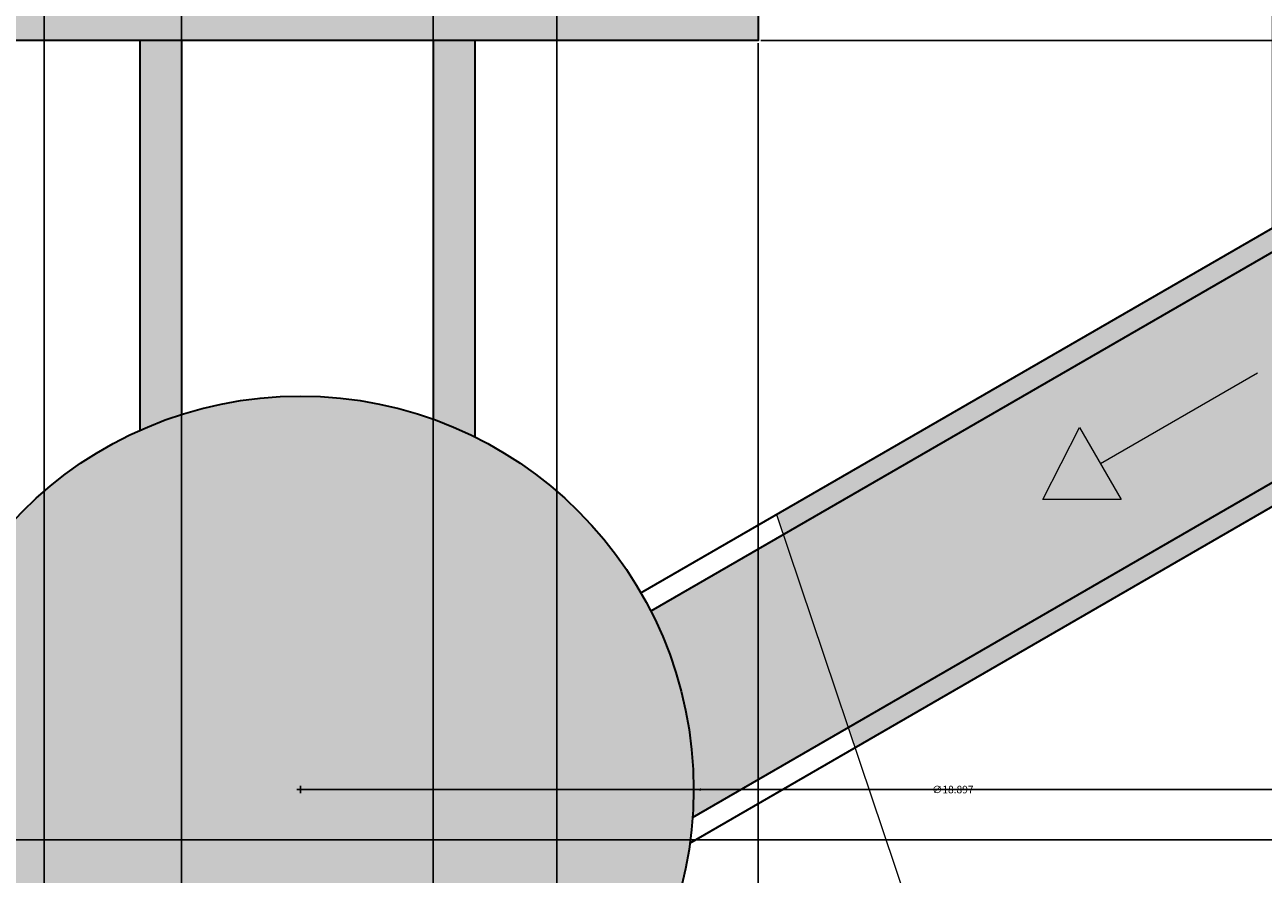
# Model space of a CAD drawing. Units: inches. Extents: x -1 to 292, y -3 to 199.
# Tile 44 of 52: x 237 to 267, y 43 to 63. Entities that reach past the tile are written whole.
import ezdxf

# ---------------------------------------------------------------- set-up
doc = ezdxf.new("R2010")
doc.units = ezdxf.units.IN
doc.header["$MEASUREMENT"] = 0
for name, color, linetype, lineweight in [('M-ANNO-LEAD', 2, 'Continuous', 18), ('M-ANNO-SYMB', 1, 'Continuous', 18), ('M-DIMS', 2, 'Continuous', 18), ('M-EQPM', 7, 'Continuous', 35), ('M-PATT', 8, 'Continuous', 13)]:
    doc.layers.add(name, color=color, linetype=linetype, lineweight=lineweight)
doc.styles.get("Standard").update_dxf_attribs({"font": 'arial.ttf'})
doc.dimstyles.get("Standard").update_dxf_attribs({"dimtxt": 0.18, "dimasz": 0.18, "dimexe": 0.18, "dimexo": 0.0625, "dimgap": 0.09, "dimtad": 0, "dimtih": 1, "dimtoh": 1, "dimdec": 4, "dimzin": 0, "dimdsep": 46, "dimtxsty": 'Standard', "dimcen": 0.09, "dimadec": 0, "dimazin": 0, "dimtfac": 1, "dimtdec": 4, "dimtofl": 0, "dimtmove": 0, "dimatfit": 3, "dimfxl": 1, "dimtolj": 1, "dimtzin": 0, "dimarcsym": 0})

# ---------------------------------------------------------------- blocks, each defined once
blk = doc.blocks.new('FLOW-ARROW-WATER')
blk.add_line((223.29, 53.741), (227.063, 51.564))
blk.add_lwpolyline([(222.79, 52.875), (221.849, 54.506), (223.79, 54.608)], close=True)
blk = doc.blocks.new('*D10')
at = {"layer": 'Defpoints', "color": 0, "transparency": 16777216}
for p in [(169.176, 99.774), (169.176, 43.391), (292.04, 43.391)]:
    blk.add_point(p, dxfattribs=at)
at = {"layer": 'M-DIMS', "color": 0, "lineweight": -2, "transparency": 16777216}
for p, q in [((169.239, 99.774), (292.22, 99.774)), ((292.04, 99.594), (292.04, 71.764)), ((292.04, 43.571), (292.04, 71.4)), ((169.239, 43.391), (292.22, 43.391))]:
    blk.add_line(p, q, dxfattribs=at)
at = {"layer": 'M-DIMS', "color": 0, "transparency": 16777216}
for points in [[(292.01, 99.594), (292.07, 99.594), (292.04, 99.774)], [(292.01, 43.571), (292.07, 43.571), (292.04, 43.391)]]:
    blk.add_solid(points, dxfattribs=at)
at = {"layer": 'M-DIMS', "color": 0, "transparency": 16777216, "insert": (292.04, 71.582), "char_height": 0.18, "attachment_point": 5}
blk.add_mtext('\\A1;56.38', dxfattribs=at)
blk = doc.blocks.new('*D25')
at = {"layer": 'Defpoints', "color": 0, "transparency": 16777216}
for p in [(273.066, 88.419), (215.241, 88.13), (273.066, -2.71)]:
    blk.add_point(p, dxfattribs=at)
at = {"layer": 'M-DIMS', "color": 0, "lineweight": -2, "transparency": 16777216}
for p, q in [((273.066, 88.357), (273.066, -2.89)), ((215.241, 88.068), (215.241, -2.89)), ((215.421, -2.71), (243.76, -2.71)), ((272.886, -2.71), (244.547, -2.71))]:
    blk.add_line(p, q, dxfattribs=at)
at = {"layer": 'M-DIMS', "color": 0, "transparency": 16777216}
for points in [[(215.421, -2.68), (215.421, -2.74), (215.241, -2.71)], [(272.886, -2.68), (272.886, -2.74), (273.066, -2.71)]]:
    blk.add_solid(points, dxfattribs=at)
at = {"layer": 'M-DIMS', "color": 0, "transparency": 16777216, "insert": (244.153, -2.71), "char_height": 0.18, "attachment_point": 5}
blk.add_mtext('\\A1;57.83', dxfattribs=at)
blk = doc.blocks.new('*D28')
at = {"layer": 'Defpoints', "color": 0, "transparency": 16777216}
for p in [(241.044, 80.582), (247.095, 80.582), (247.095, -2.71)]:
    blk.add_point(p, dxfattribs=at)
at = {"layer": 'M-DIMS', "color": 0, "lineweight": -2, "transparency": 16777216}
for p, q in [((241.044, 80.52), (241.044, -2.89)), ((247.095, 80.52), (247.095, -2.89)), ((241.224, -2.71), (243.692, -2.71)), ((246.915, -2.71), (244.446, -2.71))]:
    blk.add_line(p, q, dxfattribs=at)
at = {"layer": 'M-DIMS', "color": 0, "transparency": 16777216}
for points in [[(241.224, -2.68), (241.224, -2.74), (241.044, -2.71)], [(246.915, -2.68), (246.915, -2.74), (247.095, -2.71)]]:
    blk.add_solid(points, dxfattribs=at)
at = {"layer": 'M-DIMS', "color": 0, "transparency": 16777216, "insert": (244.069, -2.71), "char_height": 0.18, "attachment_point": 5}
blk.add_mtext('\\A1;6.051', dxfattribs=at)
blk = doc.blocks.new('*D29')
at = {"layer": 'Defpoints', "color": 0, "transparency": 16777216}
for p in [(243.903, 98.567), (243.903, 44.598), (292.04, 44.598)]:
    blk.add_point(p, dxfattribs=at)
at = {"layer": 'M-DIMS', "color": 0, "lineweight": -2, "transparency": 16777216}
for p, q in [((243.966, 98.567), (292.22, 98.567)), ((292.04, 98.387), (292.04, 71.764)), ((292.04, 44.778), (292.04, 71.4)), ((243.966, 44.598), (292.22, 44.598))]:
    blk.add_line(p, q, dxfattribs=at)
at = {"layer": 'M-DIMS', "color": 0, "transparency": 16777216}
for points in [[(292.01, 98.387), (292.07, 98.387), (292.04, 98.567)], [(292.01, 44.778), (292.07, 44.778), (292.04, 44.598)]]:
    blk.add_solid(points, dxfattribs=at)
at = {"layer": 'M-DIMS', "color": 0, "transparency": 16777216, "insert": (292.04, 71.582), "char_height": 0.18, "attachment_point": 5}
blk.add_mtext('\\A1;53.97', dxfattribs=at)
blk = doc.blocks.new('*D30')
at = {"layer": 'Defpoints', "color": 0, "transparency": 16777216}
for p in [(232.903, 62.582), (254.903, 62.582), (254.903, -2.71)]:
    blk.add_point(p, dxfattribs=at)
at = {"layer": 'M-DIMS', "color": 0, "lineweight": -2, "transparency": 16777216}
for p, q in [((232.903, 62.52), (232.903, -2.89)), ((254.903, 62.52), (254.903, -2.89)), ((233.083, -2.71), (243.684, -2.71)), ((254.723, -2.71), (244.123, -2.71))]:
    blk.add_line(p, q, dxfattribs=at)
at = {"layer": 'M-DIMS', "color": 0, "transparency": 16777216}
for points in [[(233.083, -2.68), (233.083, -2.74), (232.903, -2.71)], [(254.723, -2.68), (254.723, -2.74), (254.903, -2.71)]]:
    blk.add_solid(points, dxfattribs=at)
at = {"layer": 'M-DIMS', "color": 0, "transparency": 16777216, "insert": (243.903, -2.71), "char_height": 0.18, "attachment_point": 5}
blk.add_mtext('\\A1;22', dxfattribs=at)
blk = doc.blocks.new('*D31')
at = {"layer": 'Defpoints', "color": 0, "transparency": 16777216}
for p in [(254.903, 80.582), (292.04, 80.582), (254.903, 62.582)]:
    blk.add_point(p, dxfattribs=at)
at = {"layer": 'M-DIMS', "color": 0, "lineweight": -2, "transparency": 16777216}
for p, q in [((254.966, 80.582), (292.22, 80.582)), ((292.04, 80.402), (292.04, 71.764)), ((292.04, 62.762), (292.04, 71.4)), ((254.966, 62.582), (292.22, 62.582))]:
    blk.add_line(p, q, dxfattribs=at)
at = {"layer": 'M-DIMS', "color": 0, "transparency": 16777216}
for points in [[(292.01, 80.402), (292.07, 80.402), (292.04, 80.582)], [(292.01, 62.762), (292.07, 62.762), (292.04, 62.582)]]:
    blk.add_solid(points, dxfattribs=at)
at = {"layer": 'M-DIMS', "color": 0, "transparency": 16777216, "insert": (292.04, 71.582), "char_height": 0.18, "attachment_point": 5}
blk.add_mtext('\\A1;18', dxfattribs=at)
blk = doc.blocks.new('*D32')
at = {"layer": 'Defpoints', "color": 0, "transparency": 16777216}
for p in [(237.744, 67.423), (250.063, 67.423), (250.063, -2.71)]:
    blk.add_point(p, dxfattribs=at)
at = {"layer": 'M-DIMS', "color": 0, "lineweight": -2, "transparency": 16777216}
for p, q in [((237.744, 67.36), (237.744, -2.89)), ((250.063, 67.36), (250.063, -2.89)), ((237.924, -2.71), (243.448, -2.71)), ((249.883, -2.71), (244.359, -2.71))]:
    blk.add_line(p, q, dxfattribs=at)
at = {"layer": 'M-DIMS', "color": 0, "transparency": 16777216}
for points in [[(237.924, -2.68), (237.924, -2.74), (237.744, -2.71)], [(249.883, -2.68), (249.883, -2.74), (250.063, -2.71)]]:
    blk.add_solid(points, dxfattribs=at)
at = {"layer": 'M-DIMS', "color": 0, "transparency": 16777216, "insert": (243.903, -2.71), "char_height": 0.18, "attachment_point": 5}
blk.add_mtext('\\A1;12.319', dxfattribs=at)
blk = doc.blocks.new('*D33')
at = {"layer": 'Defpoints', "color": 0, "transparency": 16777216}
for p in [(242.955, 125.727), (292.04, 125.727), (237.933, 30.73)]:
    blk.add_point(p, dxfattribs=at)
at = {"layer": 'M-DIMS', "color": 0, "lineweight": -2, "transparency": 16777216}
for p, q in [((243.018, 125.727), (292.22, 125.727)), ((292.04, 125.547), (292.04, 78.41)), ((292.04, 30.91), (292.04, 78.046)), ((237.996, 30.73), (292.22, 30.73))]:
    blk.add_line(p, q, dxfattribs=at)
at = {"layer": 'M-DIMS', "color": 0, "transparency": 16777216}
for points in [[(292.01, 125.547), (292.07, 125.547), (292.04, 125.727)], [(292.01, 30.91), (292.07, 30.91), (292.04, 30.73)]]:
    blk.add_solid(points, dxfattribs=at)
at = {"layer": 'M-DIMS', "color": 0, "transparency": 16777216, "insert": (292.04, 78.228), "char_height": 0.18, "attachment_point": 5}
blk.add_mtext('\\A1;95', dxfattribs=at)
blk = doc.blocks.new('*D36')
at = {"layer": 'Defpoints', "color": 0, "transparency": 16777216}
for p in [(234.455, 44.597), (253.352, 44.598)]:
    blk.add_point(p, dxfattribs=at)
at = {"layer": 'M-DIMS', "color": 0, "lineweight": -2, "transparency": 16777216}
for p, q in [((243.903, 44.508), (243.903, 44.688)), ((243.813, 44.598), (243.993, 44.598)), ((259.021, 44.598), (253.532, 44.598))]:
    blk.add_line(p, q, dxfattribs=at)
at = {"layer": 'M-DIMS', "color": 0, "transparency": 16777216}
blk.add_solid([(253.532, 44.628), (253.532, 44.568), (253.352, 44.598)], dxfattribs=at)
at = {"layer": 'M-DIMS', "color": 0, "transparency": 16777216, "insert": (259.582, 44.598), "char_height": 0.18, "attachment_point": 5}
blk.add_mtext('\\A1;∅18.897', dxfattribs=at)

msp = doc.modelspace()

# ---------------------------------------------------------------- hatches: boundary and pattern name
at = {"layer": 'M-PATT'}
h = msp.add_hatch(color=256, dxfattribs=at)
h.set_gradient(color1=(0, 255, 255), color2=(0, 255, 255), tint=1, name='CYLINDER')
h.paths.add_polyline_path([(256.8092, 99.5764), (256.4077, 99.3157), (253.7155, 100.87), (251.3221, 99.3157), (248.6299, 100.87), (246.2365, 99.3157), (243.5443, 100.87), (241.1509, 99.3157), (238.4587, 100.87), (236.4209, 99.5466), (236.4209, 97.1861), (234.9209, 97.1861), (234.9209, 99.9764), (233.3731, 100.87), (230.9797, 99.3157, 1.0704128)])
h.paths.add_polyline_path([(234.4549, 44.5975, 1), (253.3518, 44.5975, 1)])
h.paths.add_polyline_path([(235.4822, 48.8821), (220.034, 57.8011), (220.034, 85.363), (232.4507, 92.5318, -0.0853739), (231.0925, 96.7051), (215.7407, 87.8418), (215.7407, 55.3224), (234.4552, 44.5176, -0.0021162), (234.4549, 44.5975, -0.1182098)])
h.paths.add_polyline_path([(222.7904, 52.8755), (221.8492, 54.5058), (223.7904, 54.6075)], flags=16)
h.paths.add_polyline_path([(216.828, 66.8912), (217.7692, 68.5216), (218.828, 66.8912)], flags=16)
h.paths.add_polyline_path([(216.8084, 83.826), (217.7497, 85.4564), (218.8084, 83.826)], flags=16)
h.paths.add_polyline_path([(226.468, 92.8803), (228.3442, 93.0348), (227.6068, 91.2362)], flags=16)
h.paths.add_polyline_path([(272.5659, 88.1304), (260.2765, 95.2257), (259.0113, 93.0196), (263.0639, 91.1046), (263.4912, 92.0087), (264.5631, 90.4612), (262.6367, 90.2004), (263.0639, 91.1046), (259.0113, 93.0196), (257.8918, 91.0677), (267.7726, 85.363), (267.7726, 57.8011), (255.5043, 50.718), (257.0663, 46.085), (272.5659, 55.0337)])
h.paths.add_polyline_path([(263.6286, 51.5636), (261.7461, 51.5636), (262.6286, 53.2956)], flags=16)
h.paths.add_polyline_path([(269.8773, 65.3608), (268.8186, 66.9911), (270.8186, 66.9911)], flags=16)
h.paths.add_polyline_path([(269.8773, 80.8843), (268.8186, 82.5146), (270.8186, 82.5146)], flags=16)
h.paths.add_polyline_path([(255.5043, 50.718), (252.3244, 48.8821, -0.1182098), (253.3518, 44.5975, -0.0177685), (253.3279, 43.9266), (257.0663, 46.085)])
h.paths.add_polyline_path([(260.2765, 95.2257), (256.7809, 97.2439, -0.0959457), (255.356, 92.5318), (257.8918, 91.0677)])
h = msp.add_hatch(color=256, dxfattribs=at)
h.set_gradient(color1=(76, 38, 47), color2=(76, 38, 47), tint=1, name='CYLINDER')
h.paths.add_polyline_path([(267.2726, 58.0898), (255.3414, 51.2013), (255.5043, 50.718), (267.7726, 57.8011), (267.7726, 85.363), (257.8918, 91.0677), (257.643, 90.634), (267.2726, 85.0743)])
h.paths.add_polyline_path([(272.5659, 55.0337), (257.0663, 46.085), (257.2293, 45.6017), (273.0659, 54.745), (273.0659, 88.4191), (260.5253, 95.6595), (260.2765, 95.2257), (272.5659, 88.1304)])
h.paths.add_polyline_path([(215.2407, 55.0337), (234.4787, 43.9266, -0.0156517), (234.4552, 44.5176), (215.7407, 55.3224), (215.7407, 87.8418), (231.0925, 96.7051, -0.0104859), (231.0257, 97.2439), (215.2407, 88.1304)])
h.paths.add_polyline_path([(220.034, 57.8011), (235.4822, 48.8821, -0.0132367), (235.7207, 49.3218), (220.534, 58.0898), (220.534, 85.0743), (232.6923, 92.0939, -0.0096587), (232.4507, 92.5318), (220.034, 85.363)])
h = msp.add_hatch(color=256, dxfattribs=at)
h.set_gradient(color1=(0, 0, 255), color2=(0, 0, 255), tint=1, name='CYLINDER')
h.paths.add_polyline_path([(227.6068, 91.2362), (228.3442, 93.0348), (226.468, 92.8803)])
h.paths.add_polyline_path([(218.8084, 83.826), (217.7497, 85.4564), (216.8084, 83.826)])
h.paths.add_polyline_path([(262.6367, 90.2004), (264.5631, 90.4612), (263.4912, 92.0087)])
h.paths.add_polyline_path([(217.7692, 68.5216), (216.828, 66.8912), (218.828, 66.8912)])
h.paths.add_polyline_path([(223.7904, 54.6075), (221.8492, 54.5058), (222.7904, 52.8755)])
h.paths.add_polyline_path([(262.6286, 53.2956), (261.7461, 51.5636), (263.6286, 51.5636)])
h.paths.add_polyline_path([(268.8186, 82.5146), (269.8773, 80.8843), (270.8186, 82.5146)])
h.paths.add_polyline_path([(268.8186, 66.9911), (269.8773, 65.3608), (270.8186, 66.9911)])
h = msp.add_hatch(color=256, dxfattribs=at)
h.set_gradient(color1=(0, 255, 255), color2=(0, 255, 255), tint=1, name='CYLINDER')
h.paths.add_polyline_path([(241.0437, 75.7414), (240.0437, 75.7414), (240.0437, 67.4228), (241.0437, 67.4228)])
h.paths.add_polyline_path([(241.0437, 62.5821), (240.0437, 62.5821), (240.0437, 53.2217, -0.0283388), (241.0437, 53.6028)])
h.paths.add_polyline_path([(241.0437, 85.9411, -0.0200063), (240.0437, 86.21), (240.0437, 80.5821), (241.0437, 80.5821)])
h.paths.add_polyline_path([(248.0947, 86.3186, -0.0201581), (247.0947, 86.0208), (247.0947, 80.5821), (248.0947, 80.5821)])
h.paths.add_polyline_path([(244.5758, 75.7414), (243.5758, 75.7414), (243.5758, 67.4228), (244.5758, 67.4228)])
h.paths.add_polyline_path([(248.0947, 75.7414), (247.0947, 75.7414), (247.0947, 67.4228), (248.0947, 67.4228)])
h.paths.add_polyline_path([(248.0947, 62.5821), (247.0947, 62.5821), (247.0947, 53.4907, -0.0287763), (248.0947, 53.0654)])
h = msp.add_hatch(color=256, dxfattribs=at)
h.set_gradient(color1=(242, 103, 34), color2=(242, 103, 34), tint=1, name='CYLINDER')
h.paths.add_polyline_path([(232.9033, 62.5821), (254.9033, 62.5821), (254.9033, 80.5821), (251.8779, 80.5821), (250.2521, 77.7473), (252.0686, 77.7473), (252.0686, 65.4168), (235.7381, 65.4168), (235.7381, 77.7473), (250.2521, 77.7473), (251.8779, 80.5821), (232.9033, 80.5821)])

# ---------------------------------------------------------------- linework, layer by layer
at = {"layer": 'M-ANNO-LEAD'}
msp.add_line((255.3414, 51.2013), (259.5359, 38.7603), dxfattribs=at)
at = {"layer": 'M-EQPM'}
for p, q in [((240.0437, 62.5821), (240.0437, 53.2217)), ((241.0437, 62.5821), (241.0437, 53.6028)), ((247.0947, 62.5821), (247.0947, 53.4907)), ((248.0947, 62.5821), (248.0947, 53.0654))]:
    msp.add_line(p, q, dxfattribs=at)
for points in [[(253.2639, 43.3124), (273.0659, 54.745), (273.0659, 88.4191), (256.8257, 97.7954)], [(253.3279, 43.9266), (272.5659, 55.0337), (272.5659, 88.1304), (256.7809, 97.2439)], [(252.3359, 48.8887), (267.7726, 57.8011), (267.7726, 85.363), (255.356, 92.5318)], [(252.0859, 49.3218), (267.2726, 58.0898), (267.2726, 85.0743), (255.1143, 92.0939)]]:
    msp.add_lwpolyline(points, dxfattribs=at)
msp.add_lwpolyline([(232.9033, 80.5821), (254.9033, 80.5821), (254.9033, 62.5821), (232.9033, 62.5821)], close=True, dxfattribs=at)
msp.add_circle((243.9033, 44.5975), 9.4484, dxfattribs=at)

# ---------------------------------------------------------------- block references
at = {"layer": 'M-ANNO-SYMB', "rotation": 60.00000000000021}
msp.add_blockref('FLOW-ARROW-WATER', (198.0249, -167.8163), dxfattribs=at)

# ---------------------------------------------------------------- dimensions: what is measured, and where the dimension line sits
at = {"layer": 'M-DIMS'}
for base, p1, p2, override, picture, middle in [((292.0399, 125.7269), (237.9333, 30.7296), (242.9552, 125.7269), {"dimdec": 0, "dimlfac": 1, "dimrnd": 0, "dimzin": 0, "dimdsep": 46, "dimlunit": 2}, '*D33', (292.0399, 78.2282)), ((292.0399, 43.3906), (169.176, 99.7735), (169.176, 43.3906), {"dimdec": 2, "dimlfac": 1, "dimrnd": 0, "dimzin": 0, "dimdsep": 46, "dimlunit": 2}, '*D10', (292.0399, 71.5821)), ((292.0399, 44.5975), (243.9033, 98.5666), (243.9033, 44.5975), {"dimdec": 2, "dimlfac": 1, "dimrnd": 0, "dimzin": 0, "dimdsep": 46, "dimlunit": 2}, '*D29', (292.0399, 71.5821)), ((292.0399, 80.5821), (254.9033, 62.5821), (254.9033, 80.5821), {"dimdec": 0, "dimlfac": 1, "dimrnd": 0, "dimzin": 0, "dimdsep": 46, "dimlunit": 2}, '*D31', (292.0399, 71.5821))]:
    dim = msp.add_linear_dim(base=base, p1=p1, p2=p2, angle=90, dimstyle='Standard', override=override, dxfattribs=at)
    dim.commit()
    dim.dimension.update_dxf_attribs({"geometry": picture, "text_midpoint": middle})
for base, p1, p2, override, picture, middle in [((273.0659, -2.7104), (215.2407, 88.1304), (273.0659, 88.4191), {"dimdec": 2, "dimlfac": 1, "dimrnd": 0, "dimzin": 0, "dimdsep": 46, "dimlunit": 2}, '*D25', (244.1533, -2.7104)), ((247.0947, -2.7104), (241.0437, 80.5821), (247.0947, 80.5821), {"dimdec": 3, "dimlfac": 1, "dimrnd": 0, "dimzin": 0, "dimdsep": 46, "dimlunit": 2}, '*D28', (244.0692, -2.7104)), ((250.0626, -2.7104), (237.744, 67.4228), (250.0626, 67.4228), {"dimdec": 3, "dimlfac": 1, "dimrnd": 0, "dimzin": 0, "dimdsep": 46, "dimlunit": 2}, '*D32', (243.9033, -2.7104)), ((254.9033, -2.7104), (232.9033, 62.5821), (254.9033, 62.5821), {"dimdec": 0, "dimlfac": 1, "dimrnd": 0, "dimzin": 0, "dimdsep": 46, "dimlunit": 2}, '*D30', (243.9033, -2.7104))]:
    dim = msp.add_linear_dim(base=base, p1=p1, p2=p2, dimstyle='Standard', override=override, dxfattribs=at)
    dim.commit()
    dim.dimension.update_dxf_attribs({"geometry": picture, "text_midpoint": middle})
dim = msp.add_diameter_dim_2p(p1=(234.4549, 44.5971), p2=(253.3518, 44.598), dimstyle='Standard', override={"dimdec": 3, "dimlfac": 1, "dimrnd": 0, "dimzin": 0, "dimdsep": 46, "dimlunit": 2}, dxfattribs=at)
dim.commit()
dim.dimension.update_dxf_attribs({"geometry": '*D36', "text_midpoint": (259.0208, 44.5983), "dimtype": 163})

doc.saveas('drawing.dxf')
